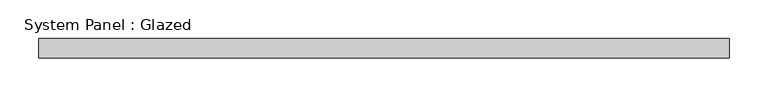
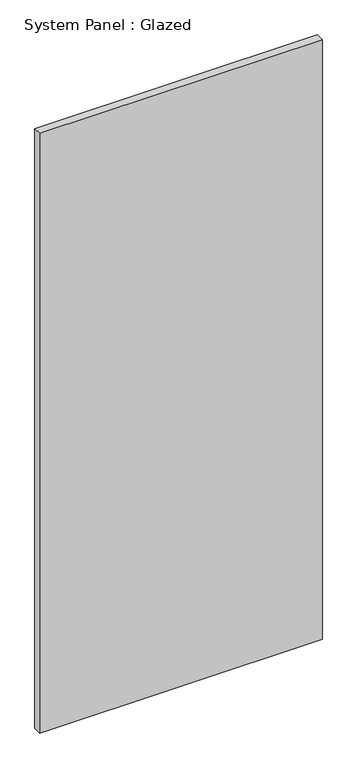
"""IFC4 building model written with IfcOpenShell, lengths in millimetres: plate geometry, System Panel : Glazed."""

from ifc_helpers import new_model, si_unit, origin, origin_with_axes, place, context, project, spatial, polyline, outline, extrude, source, transform, mapped, element, save


def system_panel_glazed_447bdfe9(model_context):
    return source(origin(), model_context, "Body", "SweptSolid", [
        extrude(outline(polyline([(447.675, 19.05), (-447.675, 19.05), (-447.675, 44.45), (447.675, 44.45), (447.675, 19.05)])), origin_with_axes(), (0.0, 0.0, 1.0), 2006.6),
    ])


if __name__ == "__main__":
    model = new_model("IFC4")
    model_context = context("Model", 3, world=origin())
    ifc_project = project(units=[si_unit("LENGTHUNIT", "METRE", prefix="MILLI")], contexts=[model_context])
    site = spatial("IfcSite", under=ifc_project)
    building = spatial("IfcBuilding", under=site)
    placement = place(None, origin())
    system_panel_glazed_shape = system_panel_glazed_447bdfe9(model_context)
    element("IfcPlate", 1, ObjectType="System Panel : Glazed", at=placement, inside=building, context=model_context, shape_type="MappedRepresentation", body=[
        mapped(system_panel_glazed_shape, transform((0.0, 0.0, 0.0), x_axis=(1.0, 0.0, 0.0), y_axis=(0.0, 1.0, 0.0), z_axis=(0.0, 0.0, 1.0))),
    ])
    save(model, "model.ifc")

# Revit data of these elements
# Type "System Panel : Glazed"
#   Construction Type Id = "GSP4R"
#   Analytic Construction = "1/8 in Pilkington single glazing"
#   Visual Light Transmittance = 0.9
#   Solar Heat Gain Coefficient = 0.86
#   Heat Transfer Coefficient (U) = 1.18115 BTU/(h·ft²·°F)
#   Define Thermal Properties by = 1
# Element 1 (IfcPlate, "System Panel : Glazed")
#   Materials on its faces: "Glass"
# Materials
#   "Glass": class "Glass", colour RGB 0 128 192, transparency 0.75, Description = "Soda Lime Glass", Cost = 0
